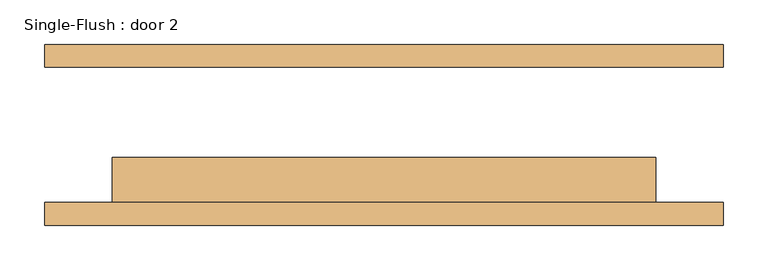
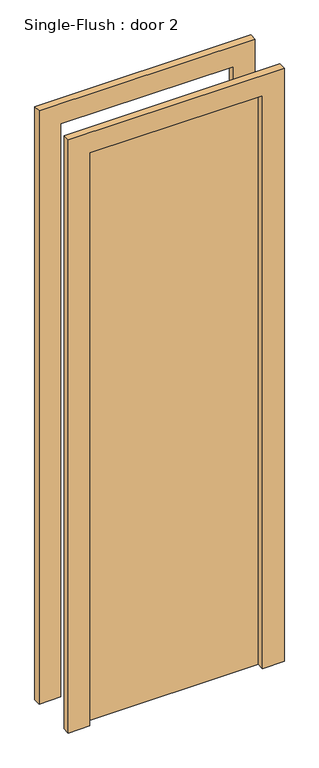
"""IFC4 building model written with IfcOpenShell, lengths in millimetres: door geometry, Single-Flush : door 2."""

from ifc_helpers import new_model, si_unit, frame, origin, origin_with_axes, place, context, project, spatial, polyline, outline, extrude, source, transform, mapped, element, save


def single_flush_door_2_5ca4d175(model_context):
    return source(origin(), model_context, "Body", "SweptSolid", [
        extrude(outline(polyline([(2209.8, -381.0), (0.0, -381.0), (0.0, -304.8), (2133.6, -304.8), (2133.6, 304.8), (0.0, 304.8), (0.0, 381.0), (2209.8, 381.0), (2209.8, -381.0)])), frame((0.0, -101.6, 0.0), z_axis=(0.0, 1.0, 0.0), x_axis=(0.0, 0.0, 1.0)), (0.0, 0.0, 1.0), 25.4),
        extrude(outline(polyline([(2209.8, 381.0), (2209.8, -381.0), (0.0, -381.0), (0.0, -304.8), (2133.6, -304.8), (2133.6, 304.8), (0.0, 304.8), (0.0, 381.0), (2209.8, 381.0)])), frame((0.0, 76.2, 0.0), z_axis=(0.0, 1.0, 0.0), x_axis=(0.0, 0.0, 1.0)), (0.0, 0.0, 1.0), 25.4),
        extrude(outline(polyline([(304.8, -25.4), (304.8, -76.2), (-304.8, -76.2), (-304.8, -25.4), (304.8, -25.4)])), origin_with_axes(), (0.0, 0.0, 1.0), 2133.6),
    ])


if __name__ == "__main__":
    model = new_model("IFC4")
    model_context = context("Model", 3, world=origin())
    ifc_project = project(units=[si_unit("LENGTHUNIT", "METRE", prefix="MILLI")], contexts=[model_context])
    site = spatial("IfcSite", under=ifc_project)
    building = spatial("IfcBuilding", under=site)
    placement = place(None, origin())
    single_flush_door_2_shape = single_flush_door_2_5ca4d175(model_context)
    element("IfcDoor", 1, ObjectType="Single-Flush : door 2", at=placement, inside=building, context=model_context, shape_type="MappedRepresentation", body=[
        mapped(single_flush_door_2_shape, transform((0.0, 0.0, 0.0), x_axis=(1.0, 0.0, 0.0), y_axis=(0.0, 1.0, 0.0), z_axis=(0.0, 0.0, 1.0))),
    ])
    save(model, "model.ifc")

# Revit data of these elements
# Type "Single-Flush : door 2"
#   Type Mark = "8"
#   Construction Type Id = "MDOOR"
#   Assembly Code = "C1020"
#   Analytic Construction = "Metal"
#   Thickness = 0' - 2"
#   Heat Transfer Coefficient (U) = 0.651978 BTU/(h·ft²·°F)
#   Height = 7' - 0"
#   Trim Projection Ext = 0' - 1"
#   Trim Projection Int = 0' - 1"
#   Trim Width = 0' - 3"
#   Width = 2' - 0"
#   Define Thermal Properties by = 1
#   Door Material = Door - Panel
#   Frame Material = Door - Frame
#   Visual Light Transmittance = 0
#   Solar Heat Gain Coefficient = 0
#   Function = (empty or 0)
#   Wall Closure = (empty or 0)
# Element 1 (IfcDoor, "Single-Flush : door 2")
#   Materials on its faces: "Door - Frame", "Door - Panel"
# Materials
#   "Door - Panel": class "Wood", colour RGB 210 159 95, transparency 0
#   "Door - Frame": colour RGB 118 70 51, transparency 0
